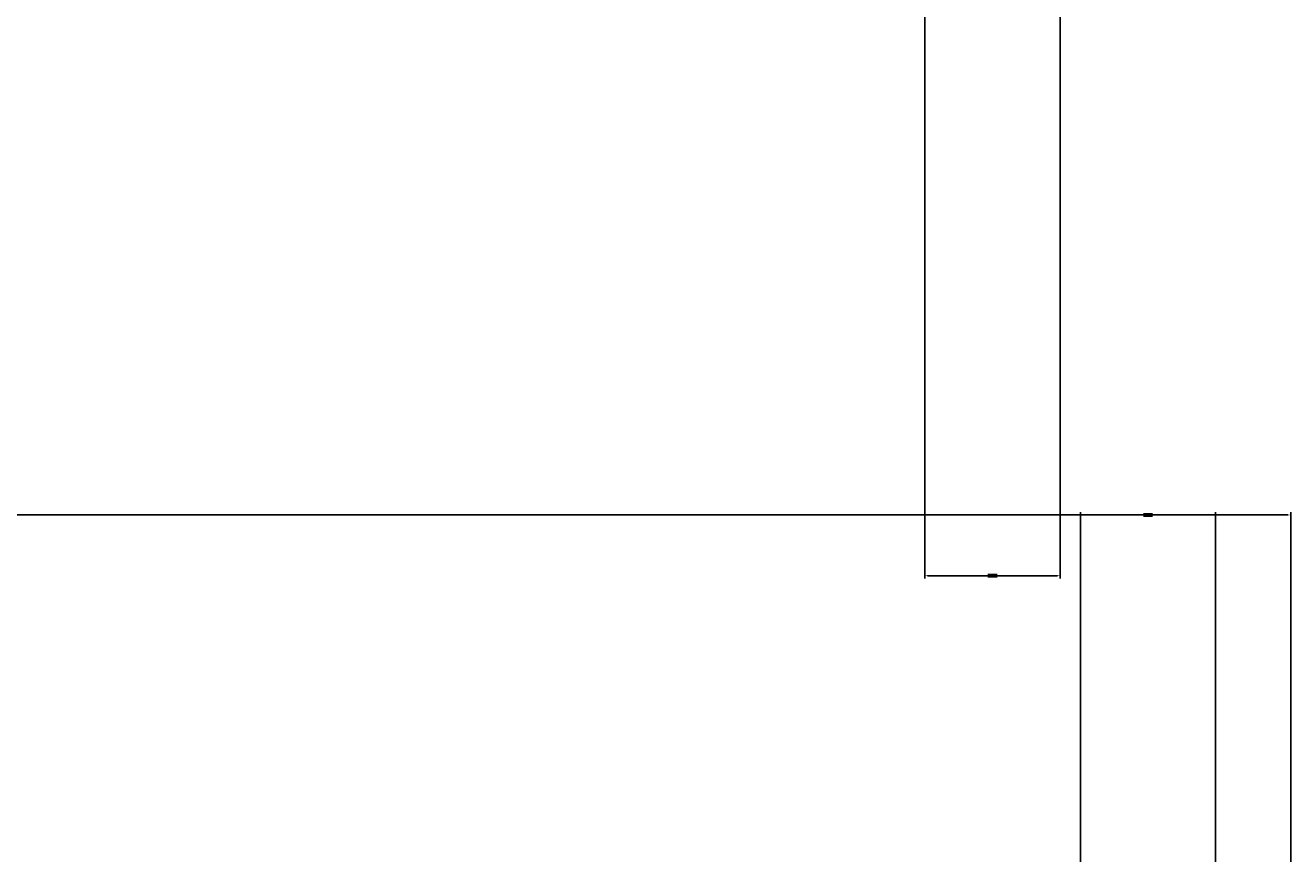
# Model space of a CAD drawing. Units: inches. Extents: x -301 to 715, y -607 to 364.
# Tile 50 of 141: x 64 to 148, y -315 to -260. Entities that reach past the tile are written whole.
import ezdxf

# ---------------------------------------------------------------- set-up
doc = ezdxf.new("R2010")
doc.units = ezdxf.units.IN
doc.header["$MEASUREMENT"] = 0
doc.layers.add('A-ANNO-DIMS', color=2, linetype='Continuous', lineweight=18)
doc.styles.get("Standard").update_dxf_attribs({"font": 'arial.ttf'})
doc.dimstyles.get("Standard").update_dxf_attribs({"dimtxt": 0.18, "dimasz": 0.18, "dimexe": 0.18, "dimexo": 0.0625, "dimgap": 0.09, "dimtad": 0, "dimtih": 1, "dimtoh": 1, "dimdec": 1, "dimzin": 0, "dimdsep": 46, "dimlunit": 4, "dimtxsty": 'Standard', "dimcen": 0.09, "dimclrd": 3, "dimclre": 4, "dimclrt": 6, "dimadec": 0, "dimazin": 0, "dimtfac": 1, "dimtdec": 1, "dimtofl": 0, "dimtmove": 0, "dimatfit": 3, "dimfxl": 1, "dimtfill": 2, "dimtfillclr": 51, "dimtolj": 1, "dimtzin": 0, "dimarcsym": 0})

# ---------------------------------------------------------------- blocks, each defined once
blk = doc.blocks.new('*D156')
at = {"layer": 'A-ANNO-DIMS', "color": 4, "lineweight": -2, "transparency": 16777216}
for p, q in [((123.897, -214.88), (123.897, -296.865)), ((132.897, -223.88), (132.897, -296.865))]:
    blk.add_line(p, q, dxfattribs=at)
at = {"layer": 'A-ANNO-DIMS', "color": 3, "lineweight": -2, "transparency": 16777216}
for p, q in [((124.077, -296.685), (128.067, -296.685)), ((132.717, -296.685), (128.726, -296.685))]:
    blk.add_line(p, q, dxfattribs=at)
at = {"layer": 'A-ANNO-DIMS', "color": 3, "transparency": 16777216}
for points in [[(124.077, -296.655), (124.077, -296.715), (123.897, -296.685)], [(132.717, -296.655), (132.717, -296.715), (132.897, -296.685)]]:
    blk.add_solid(points, dxfattribs=at)
at = {"layer": 'Defpoints', "color": 0, "transparency": 16777216}
for p in [(123.897, -214.818), (132.897, -223.818), (132.897, -296.685)]:
    blk.add_point(p, dxfattribs=at)
at = {"layer": 'A-ANNO-DIMS', "color": 6, "transparency": 16777216, "insert": (128.397, -296.685), "char_height": 0.18, "attachment_point": 5, "bg_fill": 1, "box_fill_scale": 1.25, "bg_fill_color": 51, "bg_fill_transparency": 0}
blk.add_mtext('\\A1;0\'-9"', dxfattribs=at)
blk = doc.blocks.new('*D175')
at = {"layer": 'A-ANNO-DIMS', "color": 4, "lineweight": -2, "transparency": 16777216}
for p, q in [((-199.282, -324.415), (-199.282, -292.467)), ((148.218, -324.415), (148.218, -292.467))]:
    blk.add_line(p, q, dxfattribs=at)
at = {"layer": 'A-ANNO-DIMS', "color": 3, "lineweight": -2, "transparency": 16777216}
for p, q in [((-199.102, -292.647), (-26.212, -292.647)), ((148.038, -292.647), (-24.852, -292.647))]:
    blk.add_line(p, q, dxfattribs=at)
at = {"layer": 'A-ANNO-DIMS', "color": 3, "transparency": 16777216}
for points in [[(-199.102, -292.617), (-199.102, -292.677), (-199.282, -292.647)], [(148.038, -292.617), (148.038, -292.677), (148.218, -292.647)]]:
    blk.add_solid(points, dxfattribs=at)
at = {"layer": 'Defpoints', "color": 0, "transparency": 16777216}
for p in [(148.218, -292.647), (-199.282, -324.477), (148.218, -324.477)]:
    blk.add_point(p, dxfattribs=at)
at = {"layer": 'A-ANNO-DIMS', "color": 6, "transparency": 16777216, "insert": (-25.532, -292.647), "char_height": 0.18, "attachment_point": 5, "bg_fill": 1, "box_fill_scale": 1.25, "bg_fill_color": 51, "bg_fill_transparency": 0}
blk.add_mtext('\\A1;28\'-11 1/2"', dxfattribs=at)
blk = doc.blocks.new('*D186')
at = {"layer": 'A-ANNO-DIMS', "color": 4, "lineweight": -2, "transparency": 16777216}
for p, q in [((134.255, -353.415), (134.255, -292.467)), ((143.218, -353.415), (143.218, -292.467))]:
    blk.add_line(p, q, dxfattribs=at)
at = {"layer": 'A-ANNO-DIMS', "color": 3, "lineweight": -2, "transparency": 16777216}
for p, q in [((134.435, -292.647), (138.407, -292.647)), ((143.038, -292.647), (139.066, -292.647))]:
    blk.add_line(p, q, dxfattribs=at)
at = {"layer": 'A-ANNO-DIMS', "color": 3, "transparency": 16777216}
for points in [[(134.435, -292.617), (134.435, -292.677), (134.255, -292.647)], [(143.038, -292.617), (143.038, -292.677), (143.218, -292.647)]]:
    blk.add_solid(points, dxfattribs=at)
at = {"layer": 'Defpoints', "color": 0, "transparency": 16777216}
for p in [(143.218, -292.647), (134.255, -353.477), (143.218, -353.477)]:
    blk.add_point(p, dxfattribs=at)
at = {"layer": 'A-ANNO-DIMS', "color": 6, "transparency": 16777216, "insert": (138.737, -292.647), "char_height": 0.18, "attachment_point": 5, "bg_fill": 1, "box_fill_scale": 1.25, "bg_fill_color": 51, "bg_fill_transparency": 0}
blk.add_mtext('\\A1;0\'-9"', dxfattribs=at)

msp = doc.modelspace()

# ---------------------------------------------------------------- dimensions: what is measured, and where the dimension line sits
at = {"layer": 'A-ANNO-DIMS'}
for base, p1, p2, picture, middle in [((132.897, -296.685), (123.897, -214.818), (132.897, -223.818), '*D156', (128.397, -296.685)), ((148.218, -292.647), (-199.282, -324.477), (148.218, -324.477), '*D175', (-25.532, -292.647)), ((143.218, -292.647), (134.255, -353.477), (143.218, -353.477), '*D186', (138.737, -292.647))]:
    dim = msp.add_linear_dim(base=base, p1=p1, p2=p2, dimstyle='Standard', override={"dimdec": 1, "dimlfac": 1, "dimrnd": 0, "dimzin": 1, "dimdsep": 46, "dimlunit": 4, "dimfrac": 2}, dxfattribs=at)
    dim.commit()
    dim.dimension.update_dxf_attribs({"geometry": picture, "text_midpoint": middle})

doc.saveas('drawing.dxf')
